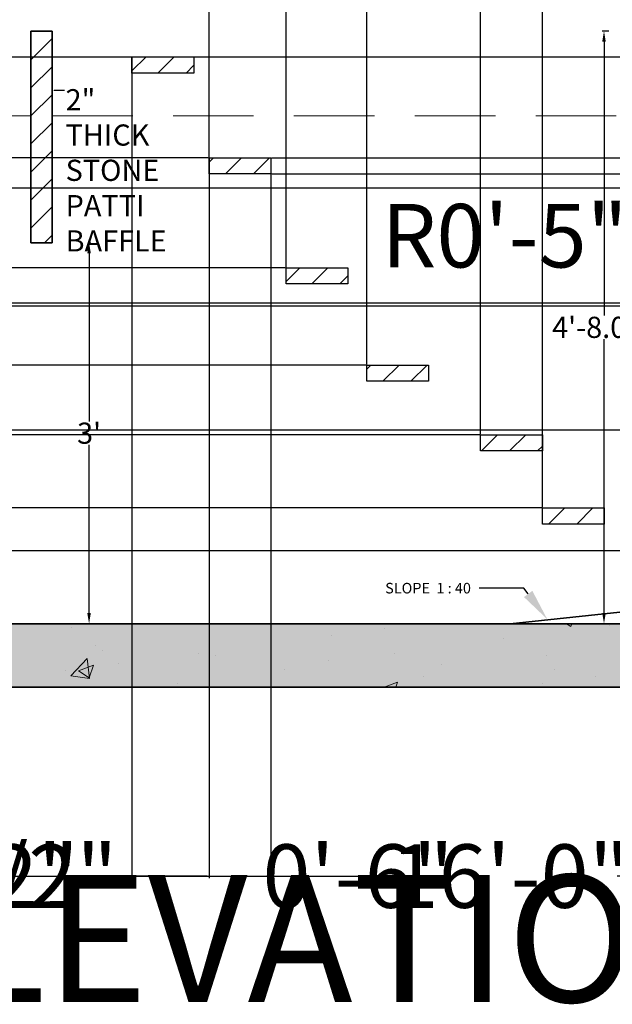
# Model space of a CAD drawing. Units: inches. Extents: x -34 to 285, y -151 to 155.
# Tile 3 of 10: x 72 to 129, y -151 to -58. Entities that reach past the tile are written whole.
import ezdxf
from ezdxf import colors
from ezdxf.entities.mleader import LeaderData, LeaderLine
from ezdxf.math import Vec2, Vec3

# ---------------------------------------------------------------- set-up
doc = ezdxf.new("R2010")
doc.units = ezdxf.units.IN
doc.header["$MEASUREMENT"] = 0
doc.linetypes.add('DASHED', pattern=[19.05, 12.7, -6.35])
for name, color, linetype, lineweight in [('A-ANNO-DIMS', 2, 'Continuous', 18), ('A-ANNO-TEXT', 7, 'Continuous', 25), ('A-DETL', 7, 'Continuous', 35), ('A-DETL-HIDN', 8, 'DASHED', 18), ('A-DETL-PATT', 8, 'Continuous', 18), ('A-FLOR-STRS', 3, 'Continuous', 25)]:
    doc.layers.add(name, color=color, linetype=linetype, lineweight=lineweight)
doc.styles.get("Standard").update_dxf_attribs({"font": 'arial.ttf'})
doc.dimstyles.get("Standard").update_dxf_attribs({"dimtxt": 6, "dimasz": 0.18, "dimexe": 0.18, "dimexo": 0.0625, "dimgap": 0.09, "dimtad": 0, "dimtih": 1, "dimtoh": 1, "dimzin": 0, "dimdsep": 46, "dimlunit": 3, "dimtxsty": 'Standard', "dimcen": 0.09, "dimadec": 0, "dimazin": 0, "dimtfac": 1, "dimtofl": 0, "dimtmove": 0, "dimatfit": 3, "dimfxl": 1, "dimtolj": 1, "dimtzin": 0, "dimarcsym": 0})

# ---------------------------------------------------------------- blocks, each defined once
blk = doc.blocks.new('*D28')
at = {"layer": 'A-ANNO-DIMS', "color": 0, "lineweight": -2, "transparency": 16777216}
for p, q in [((79.104, -78.969), (79.222, -78.969)), ((79.042, -79.969), (79.042, -95.857)), ((79.042, -113.969), (79.042, -98.081)), ((79.104, -114.969), (79.222, -114.969))]:
    blk.add_line(p, q, dxfattribs=at)
at = {"layer": 'A-ANNO-DIMS', "color": 0, "transparency": 16777216}
for points in [[(78.875, -79.969), (79.208, -79.969), (79.042, -78.969)], [(78.875, -113.969), (79.208, -113.969), (79.042, -114.969)]]:
    blk.add_solid(points, dxfattribs=at)
at = {"layer": 'Defpoints', "color": 0, "transparency": 16777216}
for p in [(79.042, -78.969), (79.042, -114.969), (79.042, -114.969)]:
    blk.add_point(p, dxfattribs=at)
at = {"layer": 'A-ANNO-DIMS', "color": 0, "transparency": 16777216, "insert": (79.042, -96.969), "char_height": 2, "attachment_point": 5}
blk.add_mtext("\\A1;3'", dxfattribs=at)
blk = doc.blocks.new('*D29')
at = {"layer": 'A-ANNO-DIMS', "color": 0, "lineweight": -2, "transparency": 16777216}
for p, q in [((128.176, -58.969), (127.544, -58.969)), ((127.724, -59.969), (127.724, -85.858)), ((127.724, -113.969), (127.724, -88.08)), ((128.176, -114.969), (127.544, -114.969))]:
    blk.add_line(p, q, dxfattribs=at)
at = {"layer": 'A-ANNO-DIMS', "color": 0, "transparency": 16777216}
for points in [[(127.557, -59.969), (127.891, -59.969), (127.724, -58.969)], [(127.557, -113.969), (127.891, -113.969), (127.724, -114.969)]]:
    blk.add_solid(points, dxfattribs=at)
at = {"layer": 'Defpoints', "color": 0, "transparency": 16777216}
for p in [(128.239, -58.969), (127.724, -114.969), (128.239, -114.969)]:
    blk.add_point(p, dxfattribs=at)
at = {"layer": 'A-ANNO-DIMS', "color": 0, "transparency": 16777216, "insert": (127.724, -86.969), "char_height": 2, "attachment_point": 5}
blk.add_mtext('\\A1;4\'-8.00"', dxfattribs=at)
blk = doc.blocks.new('*D48')
at = {"layer": 'A-ANNO-DIMS', "color": 0, "lineweight": -2, "transparency": 16777216}
for p, q in [((22.846, -121.031), (22.846, -138.999)), ((214.846, -121.031), (214.846, -138.999)), ((23.026, -138.819), (108.733, -138.819)), ((214.666, -138.819), (128.959, -138.819))]:
    blk.add_line(p, q, dxfattribs=at)
at = {"layer": 'A-ANNO-DIMS', "color": 0, "transparency": 16777216}
for points in [[(23.026, -138.789), (23.026, -138.849), (22.846, -138.819)], [(214.666, -138.789), (214.666, -138.849), (214.846, -138.819)]]:
    blk.add_solid(points, dxfattribs=at)
at = {"layer": 'Defpoints', "color": 0, "transparency": 16777216}
for p in [(22.846, -120.969), (214.846, -120.969), (214.846, -138.819)]:
    blk.add_point(p, dxfattribs=at)
at = {"layer": 'A-ANNO-DIMS', "color": 0, "transparency": 16777216, "insert": (118.846, -138.819), "char_height": 6, "attachment_point": 5}
blk.add_mtext('\\A1;16\'-0"', dxfattribs=at)
blk = doc.blocks.new('*D58')
at = {"layer": 'A-ANNO-DIMS', "color": 0, "lineweight": -2, "transparency": 16777216}
for p, q in [((83.099, -61.477), (83.099, -138.999)), ((40.846, -115.031), (40.846, -138.999)), ((41.026, -138.819), (46.919, -138.819)), ((82.919, -138.819), (77.026, -138.819))]:
    blk.add_line(p, q, dxfattribs=at)
at = {"layer": 'A-ANNO-DIMS', "color": 0, "transparency": 16777216}
for points in [[(41.026, -138.789), (41.026, -138.849), (40.846, -138.819)], [(82.919, -138.789), (82.919, -138.849), (83.099, -138.819)]]:
    blk.add_solid(points, dxfattribs=at)
at = {"layer": 'Defpoints', "color": 0, "transparency": 16777216}
for p in [(83.099, -61.415), (40.846, -114.969), (83.099, -138.819)]:
    blk.add_point(p, dxfattribs=at)
at = {"layer": 'A-ANNO-DIMS', "color": 0, "transparency": 16777216, "insert": (61.973, -138.819), "char_height": 6, "attachment_point": 5}
blk.add_mtext('\\A1;3\'-6 1/2"', dxfattribs=at)
blk = doc.blocks.new('*D59')
at = {"layer": 'A-ANNO-DIMS', "color": 0, "lineweight": -2, "transparency": 16777216}
for p, q in [((83.148, -48.969), (241.637, -48.969)), ((241.457, -49.149), (241.457, -52)), ((241.457, -61.235), (241.457, -58.384)), ((89.009, -61.415), (241.637, -61.415))]:
    blk.add_line(p, q, dxfattribs=at)
at = {"layer": 'A-ANNO-DIMS', "color": 0, "transparency": 16777216}
for points in [[(241.427, -49.149), (241.487, -49.149), (241.457, -48.969)], [(241.427, -61.235), (241.487, -61.235), (241.457, -61.415)]]:
    blk.add_solid(points, dxfattribs=at)
at = {"layer": 'Defpoints', "color": 0, "transparency": 16777216}
for p in [(83.086, -48.969), (88.947, -61.415), (241.457, -61.415)]:
    blk.add_point(p, dxfattribs=at)
at = {"layer": 'A-ANNO-DIMS', "color": 0, "transparency": 16777216, "insert": (241.457, -55.192), "char_height": 6, "attachment_point": 5}
blk.add_mtext('\\A1;1\'-0 1/2"', dxfattribs=at)
blk = doc.blocks.new('*D60')
at = {"layer": 'A-ANNO-DIMS', "color": 0, "lineweight": -2, "transparency": 16777216}
for p, q in [((90.383, -71.009), (90.383, -138.999)), ((40.846, -115.031), (40.846, -138.999)), ((41.026, -138.819), (50.439, -138.819)), ((90.203, -138.819), (80.791, -138.819))]:
    blk.add_line(p, q, dxfattribs=at)
at = {"layer": 'A-ANNO-DIMS', "color": 0, "transparency": 16777216}
for points in [[(41.026, -138.789), (41.026, -138.849), (40.846, -138.819)], [(90.203, -138.789), (90.203, -138.849), (90.383, -138.819)]]:
    blk.add_solid(points, dxfattribs=at)
at = {"layer": 'Defpoints', "color": 0, "transparency": 16777216}
for p in [(90.383, -70.947), (40.846, -114.969), (90.383, -138.819)]:
    blk.add_point(p, dxfattribs=at)
at = {"layer": 'A-ANNO-DIMS', "color": 0, "transparency": 16777216, "insert": (65.615, -138.819), "char_height": 6, "attachment_point": 5}
blk.add_mtext('\\A1;4\'-1 1/2"', dxfattribs=at)
blk = doc.blocks.new('*D64')
at = {"layer": 'A-ANNO-DIMS', "color": 0, "lineweight": -2, "transparency": 16777216}
for p, q in [((157.783, -84.969), (0.722, -84.969)), ((0.902, -85.149), (0.902, -96.816)), ((0.902, -114.789), (0.902, -103.122)), ((148.783, -114.969), (0.722, -114.969))]:
    blk.add_line(p, q, dxfattribs=at)
at = {"layer": 'A-ANNO-DIMS', "color": 0, "transparency": 16777216}
for points in [[(0.872, -85.149), (0.932, -85.149), (0.902, -84.969)], [(0.872, -114.789), (0.932, -114.789), (0.902, -114.969)]]:
    blk.add_solid(points, dxfattribs=at)
at = {"layer": 'Defpoints', "color": 0, "transparency": 16777216}
for p in [(157.846, -84.969), (0.902, -114.969), (148.846, -114.969)]:
    blk.add_point(p, dxfattribs=at)
at = {"layer": 'A-ANNO-DIMS', "color": 0, "transparency": 16777216, "insert": (0.902, -99.969), "char_height": 6, "attachment_point": 5}
blk.add_mtext('\\A1;2\'-6"', dxfattribs=at)
blk = doc.blocks.new('*D67')
at = {"layer": 'A-ANNO-DIMS', "color": 0, "lineweight": -2, "transparency": 16777216}
for p, q in [((90.321, -70.947), (0.722, -70.947)), ((0.902, -71.127), (0.902, -89.802)), ((0.902, -114.789), (0.902, -96.113)), ((118.783, -114.969), (0.722, -114.969))]:
    blk.add_line(p, q, dxfattribs=at)
at = {"layer": 'A-ANNO-DIMS', "color": 0, "transparency": 16777216}
for points in [[(0.872, -71.127), (0.932, -71.127), (0.902, -70.947)], [(0.872, -114.789), (0.932, -114.789), (0.902, -114.969)]]:
    blk.add_solid(points, dxfattribs=at)
at = {"layer": 'Defpoints', "color": 0, "transparency": 16777216}
for p in [(90.383, -70.947), (0.902, -114.969), (118.846, -114.969)]:
    blk.add_point(p, dxfattribs=at)
at = {"layer": 'A-ANNO-DIMS', "color": 0, "transparency": 16777216, "insert": (0.902, -92.958), "char_height": 6, "attachment_point": 5}
blk.add_mtext('\\A1;3\'-8"', dxfattribs=at)
blk = doc.blocks.new('*D68')
at = {"layer": 'A-ANNO-DIMS', "color": 0, "lineweight": -2, "transparency": 16777216}
for p, q in [((90.383, -70.884), (90.383, -18.978)), ((90.563, -19.158), (97.488, -19.158)), ((97.668, -81.282), (97.668, -18.978)), ((97.668, -19.158), (97.848, -19.158))]:
    blk.add_line(p, q, dxfattribs=at)
at = {"layer": 'A-ANNO-DIMS', "color": 0, "transparency": 16777216}
for points in [[(90.563, -19.128), (90.563, -19.188), (90.383, -19.158)], [(97.488, -19.128), (97.488, -19.188), (97.668, -19.158)]]:
    blk.add_solid(points, dxfattribs=at)
at = {"layer": 'Defpoints', "color": 0, "transparency": 16777216}
for p in [(97.668, -19.158), (90.383, -70.947), (97.668, -81.345)]:
    blk.add_point(p, dxfattribs=at)
at = {"layer": 'A-ANNO-DIMS', "color": 0, "transparency": 16777216, "insert": (112.903, -19.158), "char_height": 6, "attachment_point": 5}
blk.add_mtext('\\A1;0\'-7 1/2"', dxfattribs=at)
blk = doc.blocks.new('*D69')
at = {"layer": 'A-ANNO-DIMS', "color": 0, "lineweight": -2, "transparency": 16777216}
for p, q in [((97.668, -81.282), (97.668, -18.978)), ((97.848, -19.158), (105.119, -19.158)), ((105.299, -90.467), (105.299, -18.978)), ((105.299, -19.158), (105.479, -19.158))]:
    blk.add_line(p, q, dxfattribs=at)
at = {"layer": 'A-ANNO-DIMS', "color": 0, "transparency": 16777216}
for points in [[(97.848, -19.128), (97.848, -19.188), (97.668, -19.158)], [(105.119, -19.128), (105.119, -19.188), (105.299, -19.158)]]:
    blk.add_solid(points, dxfattribs=at)
at = {"layer": 'Defpoints', "color": 0, "transparency": 16777216}
for p in [(105.299, -19.158), (97.668, -81.345), (105.299, -90.53)]:
    blk.add_point(p, dxfattribs=at)
at = {"layer": 'A-ANNO-DIMS', "color": 0, "transparency": 16777216, "insert": (120.534, -19.158), "char_height": 6, "attachment_point": 5}
blk.add_mtext('\\A1;0\'-7 1/2"', dxfattribs=at)
blk = doc.blocks.new('*D70')
at = {"layer": 'A-ANNO-DIMS', "color": 0, "lineweight": -2, "transparency": 16777216}
for p, q in [((105.299, -90.467), (105.299, -18.978)), ((105.479, -19.158), (115.871, -19.158)), ((116.051, -97.053), (116.051, -18.978)), ((116.051, -19.158), (116.231, -19.158))]:
    blk.add_line(p, q, dxfattribs=at)
at = {"layer": 'A-ANNO-DIMS', "color": 0, "transparency": 16777216}
for points in [[(105.479, -19.128), (105.479, -19.188), (105.299, -19.158)], [(115.871, -19.128), (115.871, -19.188), (116.051, -19.158)]]:
    blk.add_solid(points, dxfattribs=at)
at = {"layer": 'Defpoints', "color": 0, "transparency": 16777216}
for p in [(116.051, -19.158), (105.299, -90.53), (116.051, -97.116)]:
    blk.add_point(p, dxfattribs=at)
at = {"layer": 'A-ANNO-DIMS', "color": 0, "transparency": 16777216, "insert": (126.627, -19.158), "char_height": 6, "attachment_point": 5}
blk.add_mtext('\\A1;0\'-11"', dxfattribs=at)
blk = doc.blocks.new('*D71')
at = {"layer": 'A-ANNO-DIMS', "color": 0, "lineweight": -2, "transparency": 16777216}
for p, q in [((116.051, -97.053), (116.051, -18.978)), ((116.231, -19.158), (121.719, -19.158)), ((121.899, -103.966), (121.899, -18.978)), ((121.899, -19.158), (122.079, -19.158))]:
    blk.add_line(p, q, dxfattribs=at)
at = {"layer": 'A-ANNO-DIMS', "color": 0, "transparency": 16777216}
for points in [[(116.231, -19.128), (116.231, -19.188), (116.051, -19.158)], [(121.719, -19.128), (121.719, -19.188), (121.899, -19.158)]]:
    blk.add_solid(points, dxfattribs=at)
at = {"layer": 'Defpoints', "color": 0, "transparency": 16777216}
for p in [(121.899, -19.158), (116.051, -97.116), (121.899, -104.028)]:
    blk.add_point(p, dxfattribs=at)
at = {"layer": 'A-ANNO-DIMS', "color": 0, "transparency": 16777216, "insert": (130.144, -19.158), "char_height": 6, "attachment_point": 5}
blk.add_mtext('\\A1;0\'-6"', dxfattribs=at)
blk = doc.blocks.new('*D72')
at = {"layer": 'A-ANNO-DIMS', "color": 0, "lineweight": -2, "transparency": 16777216}
for p, q in [((90.321, -70.947), (0.722, -70.947)), ((0.902, -71.127), (0.902, -72.953)), ((0.902, -81.165), (0.902, -79.338)), ((97.605, -81.345), (0.722, -81.345))]:
    blk.add_line(p, q, dxfattribs=at)
at = {"layer": 'A-ANNO-DIMS', "color": 0, "transparency": 16777216}
for points in [[(0.872, -71.127), (0.932, -71.127), (0.902, -70.947)], [(0.872, -81.165), (0.932, -81.165), (0.902, -81.345)]]:
    blk.add_solid(points, dxfattribs=at)
at = {"layer": 'Defpoints', "color": 0, "transparency": 16777216}
for p in [(90.383, -70.947), (0.902, -81.345), (97.668, -81.345)]:
    blk.add_point(p, dxfattribs=at)
at = {"layer": 'A-ANNO-DIMS', "color": 0, "transparency": 16777216, "insert": (0.902, -76.146), "char_height": 6, "attachment_point": 5}
blk.add_mtext('\\A1;0\'-10 1/2"', dxfattribs=at)
blk = doc.blocks.new('*D73')
at = {"layer": 'A-ANNO-DIMS', "color": 0, "lineweight": -2, "transparency": 16777216}
for p, q in [((97.605, -81.345), (0.722, -81.345)), ((0.902, -81.525), (0.902, -82.784)), ((0.902, -90.35), (0.902, -89.091)), ((105.236, -90.53), (0.722, -90.53))]:
    blk.add_line(p, q, dxfattribs=at)
at = {"layer": 'A-ANNO-DIMS', "color": 0, "transparency": 16777216}
for points in [[(0.872, -81.525), (0.932, -81.525), (0.902, -81.345)], [(0.872, -90.35), (0.932, -90.35), (0.902, -90.53)]]:
    blk.add_solid(points, dxfattribs=at)
at = {"layer": 'Defpoints', "color": 0, "transparency": 16777216}
for p in [(97.668, -81.345), (0.902, -90.53), (105.299, -90.53)]:
    blk.add_point(p, dxfattribs=at)
at = {"layer": 'A-ANNO-DIMS', "color": 0, "transparency": 16777216, "insert": (0.902, -85.937), "char_height": 6, "attachment_point": 5}
blk.add_mtext('\\A1;0\'-9"', dxfattribs=at)
blk = doc.blocks.new('*D74')
at = {"layer": 'A-ANNO-DIMS', "color": 0, "lineweight": -2, "transparency": 16777216}
for p, q in [((0.902, -90.35), (0.902, -90.17)), ((105.236, -90.53), (0.722, -90.53)), ((115.989, -97.116), (0.722, -97.116)), ((0.902, -97.296), (0.902, -97.476))]:
    blk.add_line(p, q, dxfattribs=at)
at = {"layer": 'A-ANNO-DIMS', "color": 0, "transparency": 16777216}
for points in [[(0.872, -90.35), (0.932, -90.35), (0.902, -90.53)], [(0.872, -97.296), (0.932, -97.296), (0.902, -97.116)]]:
    blk.add_solid(points, dxfattribs=at)
at = {"layer": 'Defpoints', "color": 0, "transparency": 16777216}
for p in [(105.299, -90.53), (0.902, -97.116), (116.051, -97.116)]:
    blk.add_point(p, dxfattribs=at)
at = {"layer": 'A-ANNO-DIMS', "color": 0, "transparency": 16777216, "insert": (0.902, -93.823), "char_height": 6, "attachment_point": 5}
blk.add_mtext('\\A1;0\'-6 1/2"', dxfattribs=at)
blk = doc.blocks.new('*D75')
at = {"layer": 'A-ANNO-DIMS', "color": 0, "lineweight": -2, "transparency": 16777216}
for p, q in [((115.989, -97.116), (0.722, -97.116)), ((0.902, -97.296), (0.902, -97.419)), ((121.836, -104.028), (0.722, -104.028)), ((0.902, -103.848), (0.902, -103.725))]:
    blk.add_line(p, q, dxfattribs=at)
at = {"layer": 'A-ANNO-DIMS', "color": 0, "transparency": 16777216}
for points in [[(0.872, -97.296), (0.932, -97.296), (0.902, -97.116)], [(0.872, -103.848), (0.932, -103.848), (0.902, -104.028)]]:
    blk.add_solid(points, dxfattribs=at)
at = {"layer": 'Defpoints', "color": 0, "transparency": 16777216}
for p in [(116.051, -97.116), (0.902, -104.028), (121.899, -104.028)]:
    blk.add_point(p, dxfattribs=at)
at = {"layer": 'A-ANNO-DIMS', "color": 0, "transparency": 16777216, "insert": (0.902, -100.572), "char_height": 6, "attachment_point": 5}
blk.add_mtext('\\A1;0\'-7"', dxfattribs=at)
blk = doc.blocks.new('*D76')
at = {"layer": 'A-ANNO-DIMS', "color": 0, "lineweight": -2, "transparency": 16777216}
for p, q in [((121.836, -104.028), (0.722, -104.028)), ((0.902, -104.208), (0.902, -106.345)), ((0.902, -114.789), (0.902, -112.652)), ((118.783, -114.969), (0.722, -114.969))]:
    blk.add_line(p, q, dxfattribs=at)
at = {"layer": 'A-ANNO-DIMS', "color": 0, "transparency": 16777216}
for points in [[(0.872, -104.208), (0.932, -104.208), (0.902, -104.028)], [(0.872, -114.789), (0.932, -114.789), (0.902, -114.969)]]:
    blk.add_solid(points, dxfattribs=at)
at = {"layer": 'Defpoints', "color": 0, "transparency": 16777216}
for p in [(121.899, -104.028), (0.902, -114.969), (118.846, -114.969)]:
    blk.add_point(p, dxfattribs=at)
at = {"layer": 'A-ANNO-DIMS', "color": 0, "transparency": 16777216, "insert": (0.902, -109.499), "char_height": 6, "attachment_point": 5}
blk.add_mtext('\\A1;0\'-11"', dxfattribs=at)
blk = doc.blocks.new('*D77')
at = {"layer": 'A-ANNO-DIMS', "color": 0, "lineweight": -2, "transparency": 16777216}
for p, q in [((90.383, -72.532), (90.383, -138.999)), ((96.231, -72.532), (96.231, -138.999)), ((90.563, -138.819), (96.051, -138.819)), ((96.231, -138.819), (96.411, -138.819))]:
    blk.add_line(p, q, dxfattribs=at)
at = {"layer": 'A-ANNO-DIMS', "color": 0, "transparency": 16777216}
for points in [[(90.563, -138.789), (90.563, -138.849), (90.383, -138.819)], [(96.051, -138.789), (96.051, -138.849), (96.231, -138.819)]]:
    blk.add_solid(points, dxfattribs=at)
at = {"layer": 'Defpoints', "color": 0, "transparency": 16777216}
for p in [(90.383, -72.47), (96.231, -72.47), (96.231, -138.819)]:
    blk.add_point(p, dxfattribs=at)
at = {"layer": 'A-ANNO-DIMS', "color": 0, "transparency": 16777216, "insert": (104.476, -138.819), "char_height": 6, "attachment_point": 5}
blk.add_mtext('\\A1;0\'-6"', dxfattribs=at)
blk = doc.blocks.new('*D78')
at = {"layer": 'A-ANNO-DIMS', "color": 0, "lineweight": -2, "transparency": 16777216}
for p, q in [((96.293, -70.947), (241.637, -70.947)), ((241.457, -71.127), (241.457, -72.29)), ((96.293, -72.47), (241.637, -72.47)), ((241.457, -72.47), (241.457, -72.65)), ((241.457, -72.65), (241.277, -72.65))]:
    blk.add_line(p, q, dxfattribs=at)
at = {"layer": 'A-ANNO-DIMS', "color": 0, "transparency": 16777216}
for points in [[(241.427, -71.127), (241.487, -71.127), (241.457, -70.947)], [(241.427, -72.29), (241.487, -72.29), (241.457, -72.47)]]:
    blk.add_solid(points, dxfattribs=at)
at = {"layer": 'Defpoints', "color": 0, "transparency": 16777216}
for p in [(96.231, -70.947), (96.231, -72.47), (241.457, -72.47)]:
    blk.add_point(p, dxfattribs=at)
at = {"layer": 'A-ANNO-DIMS', "color": 0, "transparency": 16777216, "insert": (226.222, -72.65), "char_height": 6, "attachment_point": 5}
blk.add_mtext('\\A1;0\'-1 1/2"', dxfattribs=at)
blk = doc.blocks.new('*D83')
at = {"layer": 'A-ANNO-DIMS', "color": 0, "lineweight": -2, "transparency": 16777216}
for p, q in [((153.652, -61.451), (0.722, -61.451)), ((0.902, -61.631), (0.902, -64.435)), ((0.902, -73.623), (0.902, -70.819)), ((162.652, -73.803), (0.722, -73.803))]:
    blk.add_line(p, q, dxfattribs=at)
at = {"layer": 'A-ANNO-DIMS', "color": 0, "transparency": 16777216}
for points in [[(0.872, -61.631), (0.932, -61.631), (0.902, -61.451)], [(0.872, -73.623), (0.932, -73.623), (0.902, -73.803)]]:
    blk.add_solid(points, dxfattribs=at)
at = {"layer": 'Defpoints', "color": 0, "transparency": 16777216}
for p in [(153.715, -61.451), (0.902, -73.803), (162.715, -73.803)]:
    blk.add_point(p, dxfattribs=at)
at = {"layer": 'A-ANNO-DIMS', "color": 0, "transparency": 16777216, "insert": (0.902, -67.627), "char_height": 6, "attachment_point": 5}
blk.add_mtext('\\A1;1\'-0 1/2"', dxfattribs=at)
blk = doc.blocks.new('*D84')
at = {"layer": 'A-ANNO-DIMS', "color": 0, "lineweight": -2, "transparency": 16777216}
for p, q in [((162.652, -73.803), (0.722, -73.803)), ((0.902, -73.983), (0.902, -76.094)), ((0.902, -84.513), (0.902, -82.401)), ((169.24, -84.693), (0.722, -84.693))]:
    blk.add_line(p, q, dxfattribs=at)
at = {"layer": 'A-ANNO-DIMS', "color": 0, "transparency": 16777216}
for points in [[(0.872, -73.983), (0.932, -73.983), (0.902, -73.803)], [(0.872, -84.513), (0.932, -84.513), (0.902, -84.693)]]:
    blk.add_solid(points, dxfattribs=at)
at = {"layer": 'Defpoints', "color": 0, "transparency": 16777216}
for p in [(162.715, -73.803), (0.902, -84.693), (169.303, -84.693)]:
    blk.add_point(p, dxfattribs=at)
at = {"layer": 'A-ANNO-DIMS', "color": 0, "transparency": 16777216, "insert": (0.902, -79.248), "char_height": 6, "attachment_point": 5}
blk.add_mtext('\\A1;0\'-11"', dxfattribs=at)
blk = doc.blocks.new('*D85')
at = {"layer": 'A-ANNO-DIMS', "color": 0, "lineweight": -2, "transparency": 16777216}
for p, q in [((169.24, -84.693), (0.722, -84.693)), ((0.902, -84.873), (0.902, -87.539)), ((0.902, -96.513), (0.902, -93.846)), ((179.419, -96.693), (0.722, -96.693))]:
    blk.add_line(p, q, dxfattribs=at)
at = {"layer": 'A-ANNO-DIMS', "color": 0, "transparency": 16777216}
for points in [[(0.872, -84.873), (0.932, -84.873), (0.902, -84.693)], [(0.872, -96.513), (0.932, -96.513), (0.902, -96.693)]]:
    blk.add_solid(points, dxfattribs=at)
at = {"layer": 'Defpoints', "color": 0, "transparency": 16777216}
for p in [(169.303, -84.693), (0.902, -96.693), (179.482, -96.693)]:
    blk.add_point(p, dxfattribs=at)
at = {"layer": 'A-ANNO-DIMS', "color": 0, "transparency": 16777216, "insert": (0.902, -90.693), "char_height": 6, "attachment_point": 5}
blk.add_mtext('\\A1;1\'-0"', dxfattribs=at)
blk = doc.blocks.new('*D86')
at = {"layer": 'A-ANNO-DIMS', "color": 0, "lineweight": -2, "transparency": 16777216}
for p, q in [((179.419, -96.693), (0.722, -96.693)), ((0.902, -96.873), (0.902, -99.189)), ((0.902, -107.89), (0.902, -105.574)), ((187.783, -108.07), (0.722, -108.07))]:
    blk.add_line(p, q, dxfattribs=at)
at = {"layer": 'A-ANNO-DIMS', "color": 0, "transparency": 16777216}
for points in [[(0.872, -96.873), (0.932, -96.873), (0.902, -96.693)], [(0.872, -107.89), (0.932, -107.89), (0.902, -108.07)]]:
    blk.add_solid(points, dxfattribs=at)
at = {"layer": 'Defpoints', "color": 0, "transparency": 16777216}
for p in [(179.482, -96.693), (0.902, -108.07), (187.846, -108.07)]:
    blk.add_point(p, dxfattribs=at)
at = {"layer": 'A-ANNO-DIMS', "color": 0, "transparency": 16777216, "insert": (0.902, -102.381), "char_height": 6, "attachment_point": 5}
blk.add_mtext('\\A1;0\'-11 1/2"', dxfattribs=at)
blk = doc.blocks.new('*D87')
at = {"layer": 'A-ANNO-DIMS', "color": 0, "lineweight": -2, "transparency": 16777216}
for p, q in [((187.783, -108.07), (0.722, -108.07)), ((0.902, -108.25), (0.902, -108.366)), ((196.783, -114.969), (0.722, -114.969)), ((0.902, -114.789), (0.902, -114.673))]:
    blk.add_line(p, q, dxfattribs=at)
at = {"layer": 'A-ANNO-DIMS', "color": 0, "transparency": 16777216}
for points in [[(0.872, -108.25), (0.932, -108.25), (0.902, -108.07)], [(0.872, -114.789), (0.932, -114.789), (0.902, -114.969)]]:
    blk.add_solid(points, dxfattribs=at)
at = {"layer": 'Defpoints', "color": 0, "transparency": 16777216}
for p in [(187.846, -108.07), (0.902, -114.969), (196.846, -114.969)]:
    blk.add_point(p, dxfattribs=at)
at = {"layer": 'A-ANNO-DIMS', "color": 0, "transparency": 16777216, "insert": (0.902, -111.519), "char_height": 6, "attachment_point": 5}
blk.add_mtext('\\A1;0\'-7"', dxfattribs=at)
blk = doc.blocks.new('*D93')
at = {"layer": 'A-ANNO-DIMS', "color": 0, "lineweight": -2, "transparency": 16777216}
for p, q in [((129.261, -78.309), (129.441, -78.309)), ((129.441, -78.309), (131.435, -80.304)), ((135.006, -83.969), (135.186, -83.969)), ((135.096, -84.059), (135.096, -83.879))]:
    blk.add_line(p, q, dxfattribs=at)
at = {"layer": 'A-ANNO-DIMS', "color": 0, "transparency": 16777216}
blk.add_solid([(131.456, -80.283), (131.413, -80.326), (131.562, -80.432)], dxfattribs=at)
at = {"layer": 'Defpoints', "color": 0, "transparency": 16777216}
for p in [(131.562, -80.432), (135.096, -83.969)]:
    blk.add_point(p, dxfattribs=at)
at = {"layer": 'A-ANNO-DIMS', "color": 0, "transparency": 16777216, "insert": (118.326, -78.309), "char_height": 6, "attachment_point": 5}
blk.add_mtext('\\A1;R0\'-5"', dxfattribs=at)

msp = doc.modelspace()

# ---------------------------------------------------------------- hatches: boundary and pattern name
at = {"layer": 'A-DETL-PATT'}
h = msp.add_hatch(dxfattribs=at)
h.set_pattern_fill('AR-CONC', color=256, scale=0.4)
h.set_pattern_definition([(50, (0, 0), (2.86904, -0.251009), [0.3, -3.3]), (355, (0, 0), (-0.555005, 3.00877), [0.24, -2.64]), (100.4514, (0.239, -0.021), (2.314035, 2.75776), [0.25496, -2.80457]), (46.1842, (0, 0.8), (4.268965, -0.662077), [0.45, -4.95]), (96.6356, (0.3557, 0.745), (3.73865, 3.896474), [0.38244, -4.206855]), (351.1842, (0, 0.8), (3.73865, 3.896474), [0.36, -3.96]), (21, (0.4, 0.6), (2.387628, -1.610476), [0.3, -3.3]), (326, (0.4, 0.6), (0.97326, 2.9006), [0.24, -2.64]), (71.4514, (0.599, 0.4658), (3.36089, 1.290125), [0.25496, -2.80457]), (37.5, (0, 0), (0.0486394, 1.3315754), [0, -2.608, 0, -2.68, 0, -2.65]), (7.5, (0, 0), (1.052278, 1.577647), [0, -1.528, 0, -2.548, 0, -1.01]), (327.5, (-0.892, 0), (2.1352897, -0.0902195), [0, -1, 0, -3.12, 0, -4.14]), (317.5, (-1.292, 0), (2.332745, 0.40042), [0, -1.3, 0, -2.072, 0, -2.94])])
h.paths.add_polyline_path([(214.846, -48.969), (214.846, -42.969), (184.518, -42.969), (184.518, -48.969)])
h.paths.add_polyline_path([(122.241, -42.969), (122.241, -48.969), (155.156, -48.969), (155.156, -42.969)])
h.paths.add_polyline_path([(214.846, -114.969), (22.846, -114.969), (22.846, -120.969), (214.846, -120.969)])
h = msp.add_hatch(dxfattribs=at)
h.set_pattern_fill('ANSI31', color=256, scale=15)
h.paths.add_polyline_path([(75.547, -58.969), (73.547, -58.969), (73.547, -78.969), (75.547, -78.969)])
h = msp.add_hatch(dxfattribs=at)
h.set_pattern_fill('ANSI31', color=256, scale=15)
h.paths.add_polyline_path([(127.747, -104.028), (121.899, -104.028), (121.899, -105.552), (127.747, -105.552)])
h.paths.add_polyline_path([(121.899, -97.116), (116.051, -97.116), (116.051, -98.639), (121.899, -98.639)])
h.paths.add_polyline_path([(111.146, -90.53), (105.299, -90.53), (105.299, -92.053), (111.146, -92.053)])
h.paths.add_polyline_path([(103.515, -81.345), (97.668, -81.345), (97.668, -82.868), (103.515, -82.868)])
h.paths.add_polyline_path([(96.231, -70.947), (90.383, -70.947), (90.383, -72.47), (96.231, -72.47)])
h.paths.add_polyline_path([(88.947, -61.415), (83.099, -61.415), (83.099, -62.938), (88.947, -62.938)])
h = msp.add_hatch(dxfattribs=at)
h.set_pattern_fill('AR-CONC', color=256, scale=2)
h.paths.add_polyline_path([(22.846, -114.969), (22.846, -120.969), (214.846, -120.969), (214.846, -114.969)])

# ---------------------------------------------------------------- linework, layer by layer
at = {"layer": 'A-DETL'}
for p, q in [((73.547, -78.969), (73.547, -58.969)), ((73.547, -58.969), (75.547, -58.969)), ((75.547, -78.969), (75.547, -58.969)), ((73.547, -78.969), (75.547, -78.969)), ((118.846, -114.969), (139.846, -112.768)), ((22.846, -114.969), (214.846, -114.969)), ((22.846, -120.969), (214.846, -120.969))]:
    msp.add_line(p, q, dxfattribs=at)
at = {"layer": 'A-DETL-HIDN', "ltscale": 0.6}
for p, q in [((43.754, -66.969), (73.547, -66.969)), ((75.547, -66.969), (214.207, -66.969))]:
    msp.add_line(p, q, dxfattribs=at)
at = {"layer": 'A-FLOR-STRS'}
for points in [[(88.947, -62.938), (83.099, -62.938), (83.099, -61.415), (88.947, -61.415)], [(96.231, -72.47), (90.383, -72.47), (90.383, -70.947), (96.231, -70.947)], [(103.515, -82.868), (97.668, -82.868), (97.668, -81.345), (103.515, -81.345)], [(111.146, -92.053), (105.299, -92.053), (105.299, -90.53), (111.146, -90.53)], [(121.899, -98.639), (116.051, -98.639), (116.051, -97.116), (121.899, -97.116)], [(127.747, -105.552), (121.899, -105.552), (121.899, -104.028), (127.747, -104.028)]]:
    msp.add_lwpolyline(points, close=True, dxfattribs=at)

# ---------------------------------------------------------------- texts
at = {"layer": 'A-ANNO-TEXT', "insert": (-34.52, -138.72), "char_height": 12, "attachment_point": 1}
msp.add_mtext_dynamic_manual_height_columns('SECTIONAL ELEVATION OF A SEPTIC TANK ', width=509.35271, gutter_width=1, heights=[0], dxfattribs=at)

# ---------------------------------------------------------------- dimensions: what is measured, and where the dimension line sits
at = {"layer": 'A-ANNO-DIMS'}
for base, p1, p2, picture, middle in [((97.668, -19.158), (90.383, -70.947), (97.668, -81.345), '*D68', (112.903, -19.158)), ((105.299, -19.158), (97.668, -81.345), (105.299, -90.53), '*D69', (120.534, -19.158)), ((116.051, -19.158), (105.299, -90.53), (116.051, -97.116), '*D70', (126.627, -19.158)), ((121.899, -19.158), (116.051, -97.116), (121.899, -104.028), '*D71', (130.144, -19.158)), ((83.099, -138.819), (40.846, -114.969), (83.099, -61.415), '*D58', (61.973, -138.819)), ((90.383, -138.819), (40.846, -114.969), (90.383, -70.947), '*D60', (65.615, -138.819)), ((96.231, -138.819), (90.383, -72.47), (96.231, -72.47), '*D77', (104.476, -138.819)), ((214.846, -138.819), (22.846, -120.969), (214.846, -120.969), '*D48', (118.846, -138.819))]:
    dim = msp.add_linear_dim(base=base, p1=p1, p2=p2, dimstyle='Standard', override={"dimdec": 1, "dimlfac": 1, "dimrnd": 0, "dimzin": 1, "dimdsep": 46, "dimlunit": 4, "dimfrac": 2}, dxfattribs=at)
    dim.commit()
    dim.dimension.update_dxf_attribs({"geometry": picture, "text_midpoint": middle})
for base, p1, p2, override, picture, middle in [((241.457, -61.415), (83.086, -48.969), (88.947, -61.415), {"dimdec": 1, "dimlfac": 1, "dimrnd": 0, "dimzin": 1, "dimdsep": 46, "dimlunit": 4, "dimfrac": 2}, '*D59', (241.457, -55.192)), ((0.902, -73.803), (153.715, -61.451), (162.715, -73.803), {"dimdec": 1, "dimlfac": 1, "dimrnd": 0, "dimzin": 1, "dimdsep": 46, "dimlunit": 4, "dimfrac": 2}, '*D83', (0.902, -67.627)), ((127.724, -114.969), (128.239, -58.969), (128.239, -114.969), {"dimtxt": 2, "dimasz": 1, "dimclrd": 0, "dimclre": 0, "dimclrt": 0}, '*D29', (127.724, -86.969)), ((241.457, -72.47), (96.231, -70.947), (96.231, -72.47), {"dimdec": 1, "dimlfac": 1, "dimrnd": 0, "dimzin": 1, "dimdsep": 46, "dimlunit": 4, "dimfrac": 2}, '*D78', (226.222, -72.65)), ((0.902, -81.345), (90.383, -70.947), (97.668, -81.345), {"dimdec": 1, "dimlfac": 1, "dimrnd": 0, "dimzin": 1, "dimdsep": 46, "dimlunit": 4, "dimfrac": 2}, '*D72', (0.902, -76.146)), ((0.902, -114.969), (90.383, -70.947), (118.846, -114.969), {"dimdec": 1, "dimlfac": 1, "dimrnd": 0, "dimzin": 1, "dimdsep": 46, "dimlunit": 4, "dimfrac": 2}, '*D67', (0.902, -92.958)), ((0.902, -84.693), (162.715, -73.803), (169.303, -84.693), {"dimdec": 1, "dimlfac": 1, "dimrnd": 0, "dimzin": 1, "dimdsep": 46, "dimlunit": 4, "dimfrac": 2}, '*D84', (0.902, -79.248)), ((79.042, -114.969), (79.042, -78.969), (79.042, -114.969), {"dimtxt": 2, "dimasz": 1, "dimclrd": 0, "dimclre": 0, "dimclrt": 0}, '*D28', (79.042, -96.969)), ((0.902, -90.53), (97.668, -81.345), (105.299, -90.53), {"dimdec": 1, "dimlfac": 1, "dimrnd": 0, "dimzin": 1, "dimdsep": 46, "dimlunit": 4, "dimfrac": 2}, '*D73', (0.902, -85.937)), ((0.902, -97.116), (105.299, -90.53), (116.051, -97.116), {"dimdec": 1, "dimlfac": 1, "dimrnd": 0, "dimzin": 1, "dimdsep": 46, "dimlunit": 4, "dimfrac": 2}, '*D74', (0.902, -93.823)), ((0.902, -96.693), (169.303, -84.693), (179.482, -96.693), {"dimdec": 1, "dimlfac": 1, "dimrnd": 0, "dimzin": 1, "dimdsep": 46, "dimlunit": 4, "dimfrac": 2}, '*D85', (0.902, -90.693)), ((0.902, -114.969), (157.846, -84.969), (148.846, -114.969), {"dimdec": 1, "dimlfac": 1, "dimrnd": 0, "dimzin": 1, "dimdsep": 46, "dimlunit": 4, "dimfrac": 2}, '*D64', (0.902, -99.969)), ((0.902, -108.07), (179.482, -96.693), (187.846, -108.07), {"dimdec": 1, "dimlfac": 1, "dimrnd": 0, "dimzin": 1, "dimdsep": 46, "dimlunit": 4, "dimfrac": 2}, '*D86', (0.902, -102.381)), ((0.902, -104.028), (116.051, -97.116), (121.899, -104.028), {"dimdec": 1, "dimlfac": 1, "dimrnd": 0, "dimzin": 1, "dimdsep": 46, "dimlunit": 4, "dimfrac": 2}, '*D75', (0.902, -100.572)), ((0.902, -114.969), (121.899, -104.028), (118.846, -114.969), {"dimdec": 1, "dimlfac": 1, "dimrnd": 0, "dimzin": 1, "dimdsep": 46, "dimlunit": 4, "dimfrac": 2}, '*D76', (0.902, -109.499)), ((0.902, -114.969), (187.846, -108.07), (196.846, -114.969), {"dimdec": 1, "dimlfac": 1, "dimrnd": 0, "dimzin": 1, "dimdsep": 46, "dimlunit": 4, "dimfrac": 2}, '*D87', (0.902, -111.519))]:
    dim = msp.add_linear_dim(base=base, p1=p1, p2=p2, angle=90, dimstyle='Standard', override=override, dxfattribs=at)
    dim.commit()
    dim.dimension.update_dxf_attribs({"geometry": picture, "text_midpoint": middle})
dim = msp.add_radius_dim(center=(135.096, -83.969), mpoint=(131.562, -80.432), dimstyle='Standard', override={"dimdec": 1, "dimlfac": 1, "dimrnd": 0, "dimzin": 1, "dimdsep": 46, "dimlunit": 4, "dimfrac": 2}, dxfattribs=at)
dim.commit()
dim.dimension.update_dxf_attribs({"geometry": '*D93', "text_midpoint": (118.326, -78.309), "dimtype": 164})

# ---------------------------------------------------------------- leaders
at = {"layer": 'A-ANNO-TEXT'}
ml = msp.add_multileader_mtext('Standard', dxfattribs=at)
ml.set_content('{\\H11.11111x;2" THICK STONE PATTI\\P\\H1x;BAFFLE}', color=256)
ml.set_leader_properties()
ml.build(insert=Vec2(0, 0))
ml.multileader.update_dxf_attribs({"dogleg_length": 0.36, "arrow_head_size": 0.18})
ctx = ml.context
ctx.base_point, ctx.char_height, ctx.arrow_head_size, ctx.landing_gap_size, ctx.plane_origin = Vec3(76.731, -64.554), 0.18, 0.18, 0.09, Vec3(75.547, -64.554)
notes = []
notes.append((ctx, [(0, (1, 1, 0), (76.371, -64.554), (1, 0), 0.36, [(0, [(75.547, -64.554)], 0, [])])]))
ctx.mtext.insert, ctx.mtext.flow_direction = Vec3(76.821, -64.464), 5
ml = msp.add_multileader_mtext('Standard', dxfattribs=at)
ml.set_content('SLOPE  1 : 40 ', color=(248, 215, 49))
ml.set_leader_properties()
ml.build(insert=Vec2(0, 0))
ml.multileader.update_dxf_attribs({"dogleg_length": 4.22, "arrow_head_size": 3})
ctx = ml.context
ctx.base_point, ctx.char_height, ctx.arrow_head_size, ctx.landing_gap_size, ctx.plane_origin = Vec3(106.946, -111.62), 1, 3, 0.09, Vec3(122.361, -114.553)
notes.append((ctx, [(0, (1, 1, 0), (120.147, -111.62), (-1, 0), 4.22, [(0, [(122.361, -114.553)], 0, [])])]))
ctx.mtext.insert, ctx.mtext.flow_direction = Vec3(107.036, -111.111), 5
for ctx, leaders in notes:
    for number, flags, end, landing, length, lines in leaders:
        leader = LeaderData()
        leader.index, (leader.has_last_leader_line, leader.has_dogleg_vector, leader.attachment_direction) = number, flags
        leader.last_leader_point, leader.dogleg_vector, leader.dogleg_length = Vec3(end), Vec3(landing), length
        for number, points, colour, breaks in lines:
            line = LeaderLine()
            line.index, line.vertices, line.color, line.breaks = number, Vec3.list(points), colors.encode_raw_color(colour), breaks
            leader.lines.append(line)
        ctx.leaders.append(leader)

doc.saveas('drawing.dxf')
